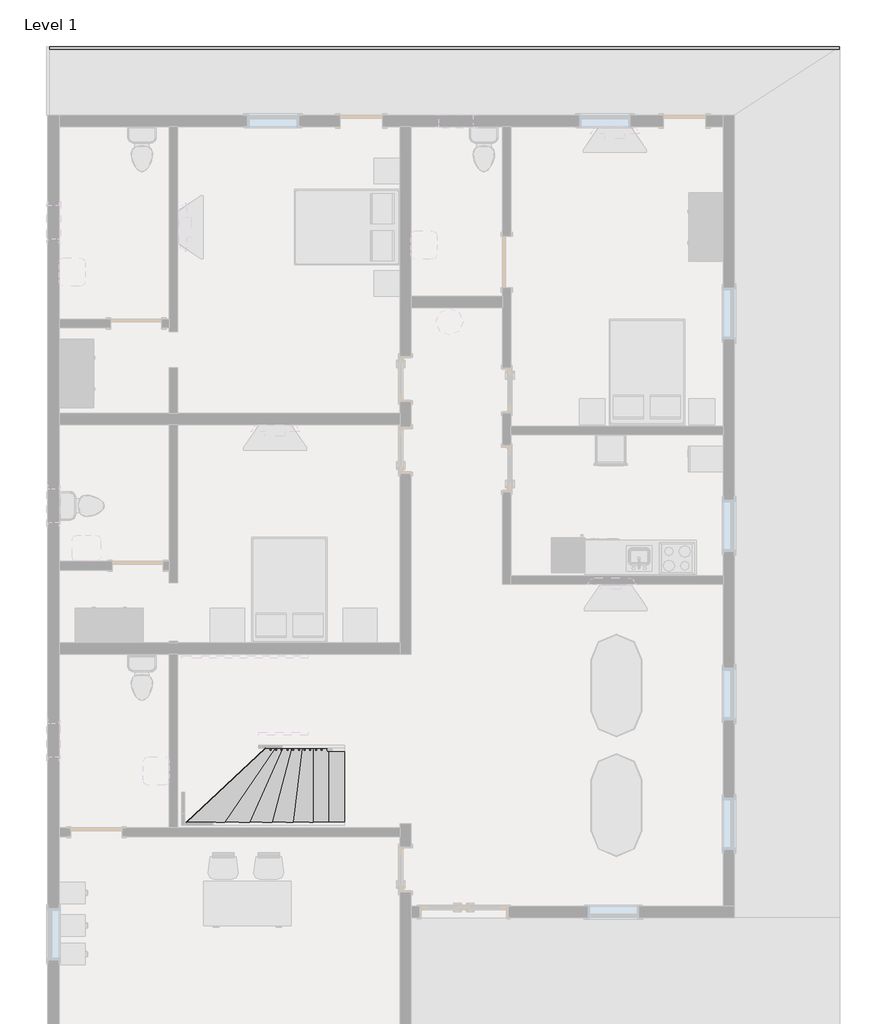
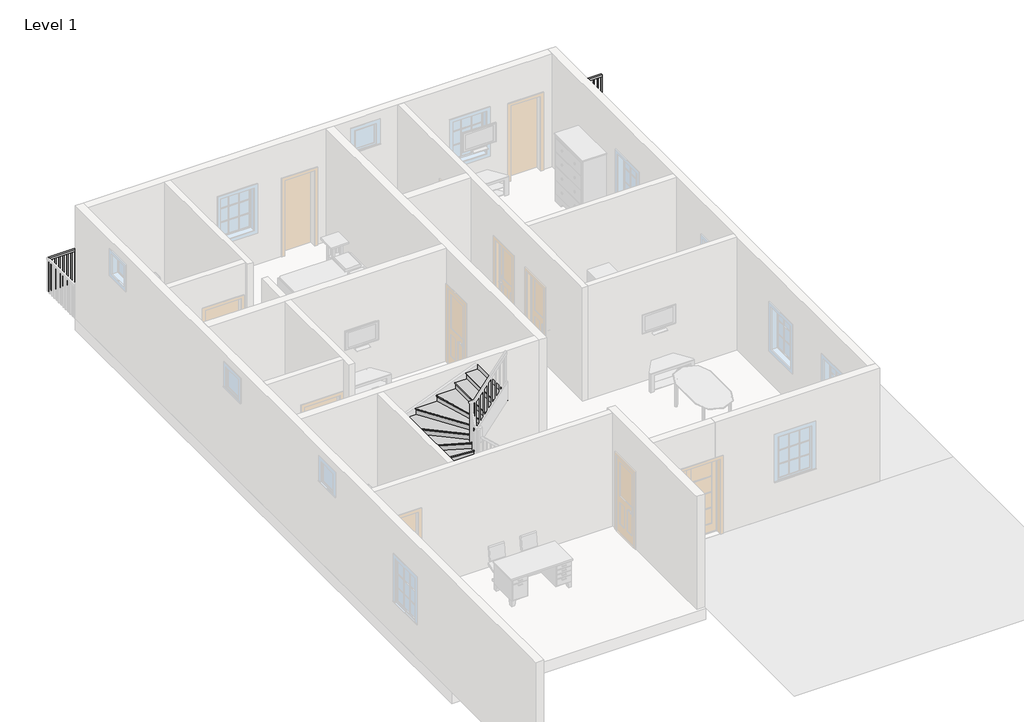
# One storey, part 3 of 4: 1 railing, 1 stair flight.
"""IFC4 building model written with IfcOpenShell, lengths in millimetres."""

from ifc_helpers import new_model, si_unit, frame, origin, origin_with_axes, place, context, project, spatial, polyline, outline, extrude, transform, mapped, element, save
from components import stair_flight_ec2dc638

model = new_model("IFC4")

# Units and contexts
model_context = context("Model", 3, world=origin())
ifc_project = project(units=[si_unit("LENGTHUNIT", "METRE", prefix="MILLI")], contexts=[model_context])

# Site, building, storey
site = spatial("IfcSite", under=ifc_project)
building = spatial("IfcBuilding", under=site)
storey = spatial("IfcBuildingStorey", under=building, Name="Level 1", Elevation=0.0)

# Railing
placement = place(None, origin())
element("IfcRailing", 1, ObjectType="Handrail - Rectangular", at=placement, inside=storey, context=model_context, shape_type="SweptSolid", body=[
    extrude(outline(polyline([(8571.673647, 10436.3488108), (8571.673647, 10385.5488108), (-5525.326353, 10385.5488108), (-5525.326353, 10436.3488108), (8571.673647, 10436.3488108)])), frame((0.0, 0.0, 863.6), z_axis=(0.0, 0.0, 1.0), x_axis=(1.0, 0.0, 0.0)), (0.0, 0.0, 1.0), 50.8),
    extrude(outline(polyline([(-5439.601353, 10420.4738108), (-5439.601353, 10401.4238108), (-5458.651353, 10401.4238108), (-5458.651353, 10420.4738108), (-5439.601353, 10420.4738108)])), origin_with_axes(), (0.0, 0.0, 1.0), 863.6),
    extrude(outline(polyline([(-5338.001353, 10420.4738108), (-5338.001353, 10401.4238108), (-5357.051353, 10401.4238108), (-5357.051353, 10420.4738108), (-5338.001353, 10420.4738108)])), origin_with_axes(), (0.0, 0.0, 1.0), 863.6),
    extrude(outline(polyline([(-5236.401353, 10420.4738108), (-5236.401353, 10401.4238108), (-5255.451353, 10401.4238108), (-5255.451353, 10420.4738108), (-5236.401353, 10420.4738108)])), origin_with_axes(), (0.0, 0.0, 1.0), 863.6),
    extrude(outline(polyline([(-5134.801353, 10420.4738108), (-5134.801353, 10401.4238108), (-5153.851353, 10401.4238108), (-5153.851353, 10420.4738108), (-5134.801353, 10420.4738108)])), origin_with_axes(), (0.0, 0.0, 1.0), 863.6),
    extrude(outline(polyline([(-5033.201353, 10420.4738108), (-5033.201353, 10401.4238108), (-5052.251353, 10401.4238108), (-5052.251353, 10420.4738108), (-5033.201353, 10420.4738108)])), origin_with_axes(), (0.0, 0.0, 1.0), 863.6),
    extrude(outline(polyline([(-4931.601353, 10420.4738108), (-4931.601353, 10401.4238108), (-4950.651353, 10401.4238108), (-4950.651353, 10420.4738108), (-4931.601353, 10420.4738108)])), origin_with_axes(), (0.0, 0.0, 1.0), 863.6),
    extrude(outline(polyline([(-4830.001353, 10420.4738108), (-4830.001353, 10401.4238108), (-4849.051353, 10401.4238108), (-4849.051353, 10420.4738108), (-4830.001353, 10420.4738108)])), origin_with_axes(), (0.0, 0.0, 1.0), 863.6),
    extrude(outline(polyline([(-4728.401353, 10420.4738108), (-4728.401353, 10401.4238108), (-4747.451353, 10401.4238108), (-4747.451353, 10420.4738108), (-4728.401353, 10420.4738108)])), origin_with_axes(), (0.0, 0.0, 1.0), 863.6),
    extrude(outline(polyline([(-4626.801353, 10420.4738108), (-4626.801353, 10401.4238108), (-4645.851353, 10401.4238108), (-4645.851353, 10420.4738108), (-4626.801353, 10420.4738108)])), origin_with_axes(), (0.0, 0.0, 1.0), 863.6),
    extrude(outline(polyline([(-4525.201353, 10420.4738108), (-4525.201353, 10401.4238108), (-4544.251353, 10401.4238108), (-4544.251353, 10420.4738108), (-4525.201353, 10420.4738108)])), origin_with_axes(), (0.0, 0.0, 1.0), 863.6),
    extrude(outline(polyline([(-4423.601353, 10420.4738108), (-4423.601353, 10401.4238108), (-4442.651353, 10401.4238108), (-4442.651353, 10420.4738108), (-4423.601353, 10420.4738108)])), origin_with_axes(), (0.0, 0.0, 1.0), 863.6),
    extrude(outline(polyline([(-4322.001353, 10420.4738108), (-4322.001353, 10401.4238108), (-4341.051353, 10401.4238108), (-4341.051353, 10420.4738108), (-4322.001353, 10420.4738108)])), origin_with_axes(), (0.0, 0.0, 1.0), 863.6),
    extrude(outline(polyline([(-4220.401353, 10420.4738108), (-4220.401353, 10401.4238108), (-4239.451353, 10401.4238108), (-4239.451353, 10420.4738108), (-4220.401353, 10420.4738108)])), origin_with_axes(), (0.0, 0.0, 1.0), 863.6),
    extrude(outline(polyline([(-4118.801353, 10420.4738108), (-4118.801353, 10401.4238108), (-4137.851353, 10401.4238108), (-4137.851353, 10420.4738108), (-4118.801353, 10420.4738108)])), origin_with_axes(), (0.0, 0.0, 1.0), 863.6),
    extrude(outline(polyline([(-4017.201353, 10420.4738108), (-4017.201353, 10401.4238108), (-4036.251353, 10401.4238108), (-4036.251353, 10420.4738108), (-4017.201353, 10420.4738108)])), origin_with_axes(), (0.0, 0.0, 1.0), 863.6),
    extrude(outline(polyline([(-3915.601353, 10420.4738108), (-3915.601353, 10401.4238108), (-3934.651353, 10401.4238108), (-3934.651353, 10420.4738108), (-3915.601353, 10420.4738108)])), origin_with_axes(), (0.0, 0.0, 1.0), 863.6),
    extrude(outline(polyline([(-3814.001353, 10420.4738108), (-3814.001353, 10401.4238108), (-3833.051353, 10401.4238108), (-3833.051353, 10420.4738108), (-3814.001353, 10420.4738108)])), origin_with_axes(), (0.0, 0.0, 1.0), 863.6),
    extrude(outline(polyline([(-3712.401353, 10420.4738108), (-3712.401353, 10401.4238108), (-3731.451353, 10401.4238108), (-3731.451353, 10420.4738108), (-3712.401353, 10420.4738108)])), origin_with_axes(), (0.0, 0.0, 1.0), 863.6),
    extrude(outline(polyline([(-3610.801353, 10420.4738108), (-3610.801353, 10401.4238108), (-3629.851353, 10401.4238108), (-3629.851353, 10420.4738108), (-3610.801353, 10420.4738108)])), origin_with_axes(), (0.0, 0.0, 1.0), 863.6),
    extrude(outline(polyline([(-3509.201353, 10420.4738108), (-3509.201353, 10401.4238108), (-3528.251353, 10401.4238108), (-3528.251353, 10420.4738108), (-3509.201353, 10420.4738108)])), origin_with_axes(), (0.0, 0.0, 1.0), 863.6),
    extrude(outline(polyline([(-3407.601353, 10420.4738108), (-3407.601353, 10401.4238108), (-3426.651353, 10401.4238108), (-3426.651353, 10420.4738108), (-3407.601353, 10420.4738108)])), origin_with_axes(), (0.0, 0.0, 1.0), 863.6),
    extrude(outline(polyline([(-3306.001353, 10420.4738108), (-3306.001353, 10401.4238108), (-3325.051353, 10401.4238108), (-3325.051353, 10420.4738108), (-3306.001353, 10420.4738108)])), origin_with_axes(), (0.0, 0.0, 1.0), 863.6),
    extrude(outline(polyline([(-3204.401353, 10420.4738108), (-3204.401353, 10401.4238108), (-3223.451353, 10401.4238108), (-3223.451353, 10420.4738108), (-3204.401353, 10420.4738108)])), origin_with_axes(), (0.0, 0.0, 1.0), 863.6),
    extrude(outline(polyline([(-3102.801353, 10420.4738108), (-3102.801353, 10401.4238108), (-3121.851353, 10401.4238108), (-3121.851353, 10420.4738108), (-3102.801353, 10420.4738108)])), origin_with_axes(), (0.0, 0.0, 1.0), 863.6),
    extrude(outline(polyline([(-3001.201353, 10420.4738108), (-3001.201353, 10401.4238108), (-3020.251353, 10401.4238108), (-3020.251353, 10420.4738108), (-3001.201353, 10420.4738108)])), origin_with_axes(), (0.0, 0.0, 1.0), 863.6),
    extrude(outline(polyline([(-2899.601353, 10420.4738108), (-2899.601353, 10401.4238108), (-2918.651353, 10401.4238108), (-2918.651353, 10420.4738108), (-2899.601353, 10420.4738108)])), origin_with_axes(), (0.0, 0.0, 1.0), 863.6),
    extrude(outline(polyline([(-2798.001353, 10420.4738108), (-2798.001353, 10401.4238108), (-2817.051353, 10401.4238108), (-2817.051353, 10420.4738108), (-2798.001353, 10420.4738108)])), origin_with_axes(), (0.0, 0.0, 1.0), 863.6),
    extrude(outline(polyline([(-2696.401353, 10420.4738108), (-2696.401353, 10401.4238108), (-2715.451353, 10401.4238108), (-2715.451353, 10420.4738108), (-2696.401353, 10420.4738108)])), origin_with_axes(), (0.0, 0.0, 1.0), 863.6),
    extrude(outline(polyline([(-2594.801353, 10420.4738108), (-2594.801353, 10401.4238108), (-2613.851353, 10401.4238108), (-2613.851353, 10420.4738108), (-2594.801353, 10420.4738108)])), origin_with_axes(), (0.0, 0.0, 1.0), 863.6),
    extrude(outline(polyline([(-2493.201353, 10420.4738108), (-2493.201353, 10401.4238108), (-2512.251353, 10401.4238108), (-2512.251353, 10420.4738108), (-2493.201353, 10420.4738108)])), origin_with_axes(), (0.0, 0.0, 1.0), 863.6),
    extrude(outline(polyline([(-2391.601353, 10420.4738108), (-2391.601353, 10401.4238108), (-2410.651353, 10401.4238108), (-2410.651353, 10420.4738108), (-2391.601353, 10420.4738108)])), origin_with_axes(), (0.0, 0.0, 1.0), 863.6),
    extrude(outline(polyline([(-2290.001353, 10420.4738108), (-2290.001353, 10401.4238108), (-2309.051353, 10401.4238108), (-2309.051353, 10420.4738108), (-2290.001353, 10420.4738108)])), origin_with_axes(), (0.0, 0.0, 1.0), 863.6),
    extrude(outline(polyline([(-2188.401353, 10420.4738108), (-2188.401353, 10401.4238108), (-2207.451353, 10401.4238108), (-2207.451353, 10420.4738108), (-2188.401353, 10420.4738108)])), origin_with_axes(), (0.0, 0.0, 1.0), 863.6),
    extrude(outline(polyline([(-2086.801353, 10420.4738108), (-2086.801353, 10401.4238108), (-2105.851353, 10401.4238108), (-2105.851353, 10420.4738108), (-2086.801353, 10420.4738108)])), origin_with_axes(), (0.0, 0.0, 1.0), 863.6),
    extrude(outline(polyline([(-1985.201353, 10420.4738108), (-1985.201353, 10401.4238108), (-2004.251353, 10401.4238108), (-2004.251353, 10420.4738108), (-1985.201353, 10420.4738108)])), origin_with_axes(), (0.0, 0.0, 1.0), 863.6),
    extrude(outline(polyline([(-1883.601353, 10420.4738108), (-1883.601353, 10401.4238108), (-1902.651353, 10401.4238108), (-1902.651353, 10420.4738108), (-1883.601353, 10420.4738108)])), origin_with_axes(), (0.0, 0.0, 1.0), 863.6),
    extrude(outline(polyline([(-1782.001353, 10420.4738108), (-1782.001353, 10401.4238108), (-1801.051353, 10401.4238108), (-1801.051353, 10420.4738108), (-1782.001353, 10420.4738108)])), origin_with_axes(), (0.0, 0.0, 1.0), 863.6),
    extrude(outline(polyline([(-1680.401353, 10420.4738108), (-1680.401353, 10401.4238108), (-1699.451353, 10401.4238108), (-1699.451353, 10420.4738108), (-1680.401353, 10420.4738108)])), origin_with_axes(), (0.0, 0.0, 1.0), 863.6),
    extrude(outline(polyline([(-1578.801353, 10420.4738108), (-1578.801353, 10401.4238108), (-1597.851353, 10401.4238108), (-1597.851353, 10420.4738108), (-1578.801353, 10420.4738108)])), origin_with_axes(), (0.0, 0.0, 1.0), 863.6),
    extrude(outline(polyline([(-1477.201353, 10420.4738108), (-1477.201353, 10401.4238108), (-1496.251353, 10401.4238108), (-1496.251353, 10420.4738108), (-1477.201353, 10420.4738108)])), origin_with_axes(), (0.0, 0.0, 1.0), 863.6),
    extrude(outline(polyline([(-1375.601353, 10420.4738108), (-1375.601353, 10401.4238108), (-1394.651353, 10401.4238108), (-1394.651353, 10420.4738108), (-1375.601353, 10420.4738108)])), origin_with_axes(), (0.0, 0.0, 1.0), 863.6),
    extrude(outline(polyline([(-1274.001353, 10420.4738108), (-1274.001353, 10401.4238108), (-1293.051353, 10401.4238108), (-1293.051353, 10420.4738108), (-1274.001353, 10420.4738108)])), origin_with_axes(), (0.0, 0.0, 1.0), 863.6),
    extrude(outline(polyline([(-1172.401353, 10420.4738108), (-1172.401353, 10401.4238108), (-1191.451353, 10401.4238108), (-1191.451353, 10420.4738108), (-1172.401353, 10420.4738108)])), origin_with_axes(), (0.0, 0.0, 1.0), 863.6),
    extrude(outline(polyline([(-1070.801353, 10420.4738108), (-1070.801353, 10401.4238108), (-1089.851353, 10401.4238108), (-1089.851353, 10420.4738108), (-1070.801353, 10420.4738108)])), origin_with_axes(), (0.0, 0.0, 1.0), 863.6),
    extrude(outline(polyline([(-969.201353, 10420.4738108), (-969.201353, 10401.4238108), (-988.251353, 10401.4238108), (-988.251353, 10420.4738108), (-969.201353, 10420.4738108)])), origin_with_axes(), (0.0, 0.0, 1.0), 863.6),
    extrude(outline(polyline([(-867.601353, 10420.4738108), (-867.601353, 10401.4238108), (-886.651353, 10401.4238108), (-886.651353, 10420.4738108), (-867.601353, 10420.4738108)])), origin_with_axes(), (0.0, 0.0, 1.0), 863.6),
    extrude(outline(polyline([(-766.001353, 10420.4738108), (-766.001353, 10401.4238108), (-785.051353, 10401.4238108), (-785.051353, 10420.4738108), (-766.001353, 10420.4738108)])), origin_with_axes(), (0.0, 0.0, 1.0), 863.6),
    extrude(outline(polyline([(-664.401353, 10420.4738108), (-664.401353, 10401.4238108), (-683.451353, 10401.4238108), (-683.451353, 10420.4738108), (-664.401353, 10420.4738108)])), origin_with_axes(), (0.0, 0.0, 1.0), 863.6),
    extrude(outline(polyline([(-562.801353, 10420.4738108), (-562.801353, 10401.4238108), (-581.851353, 10401.4238108), (-581.851353, 10420.4738108), (-562.801353, 10420.4738108)])), origin_with_axes(), (0.0, 0.0, 1.0), 863.6),
    extrude(outline(polyline([(-461.201353, 10420.4738108), (-461.201353, 10401.4238108), (-480.251353, 10401.4238108), (-480.251353, 10420.4738108), (-461.201353, 10420.4738108)])), origin_with_axes(), (0.0, 0.0, 1.0), 863.6),
    extrude(outline(polyline([(-359.601353, 10420.4738108), (-359.601353, 10401.4238108), (-378.651353, 10401.4238108), (-378.651353, 10420.4738108), (-359.601353, 10420.4738108)])), origin_with_axes(), (0.0, 0.0, 1.0), 863.6),
    extrude(outline(polyline([(-258.001353, 10420.4738108), (-258.001353, 10401.4238108), (-277.051353, 10401.4238108), (-277.051353, 10420.4738108), (-258.001353, 10420.4738108)])), origin_with_axes(), (0.0, 0.0, 1.0), 863.6),
    extrude(outline(polyline([(-156.401353, 10420.4738108), (-156.401353, 10401.4238108), (-175.451353, 10401.4238108), (-175.451353, 10420.4738108), (-156.401353, 10420.4738108)])), origin_with_axes(), (0.0, 0.0, 1.0), 863.6),
    extrude(outline(polyline([(-54.801353, 10420.4738108), (-54.801353, 10401.4238108), (-73.851353, 10401.4238108), (-73.851353, 10420.4738108), (-54.801353, 10420.4738108)])), origin_with_axes(), (0.0, 0.0, 1.0), 863.6),
    extrude(outline(polyline([(46.798647, 10420.4738108), (46.798647, 10401.4238108), (27.748647, 10401.4238108), (27.748647, 10420.4738108), (46.798647, 10420.4738108)])), origin_with_axes(), (0.0, 0.0, 1.0), 863.6),
    extrude(outline(polyline([(148.398647, 10420.4738108), (148.398647, 10401.4238108), (129.348647, 10401.4238108), (129.348647, 10420.4738108), (148.398647, 10420.4738108)])), origin_with_axes(), (0.0, 0.0, 1.0), 863.6),
    extrude(outline(polyline([(249.998647, 10420.4738108), (249.998647, 10401.4238108), (230.948647, 10401.4238108), (230.948647, 10420.4738108), (249.998647, 10420.4738108)])), origin_with_axes(), (0.0, 0.0, 1.0), 863.6),
    extrude(outline(polyline([(351.598647, 10420.4738108), (351.598647, 10401.4238108), (332.548647, 10401.4238108), (332.548647, 10420.4738108), (351.598647, 10420.4738108)])), origin_with_axes(), (0.0, 0.0, 1.0), 863.6),
    extrude(outline(polyline([(453.198647, 10420.4738108), (453.198647, 10401.4238108), (434.148647, 10401.4238108), (434.148647, 10420.4738108), (453.198647, 10420.4738108)])), origin_with_axes(), (0.0, 0.0, 1.0), 863.6),
    extrude(outline(polyline([(554.798647, 10420.4738108), (554.798647, 10401.4238108), (535.748647, 10401.4238108), (535.748647, 10420.4738108), (554.798647, 10420.4738108)])), origin_with_axes(), (0.0, 0.0, 1.0), 863.6),
    extrude(outline(polyline([(656.398647, 10420.4738108), (656.398647, 10401.4238108), (637.348647, 10401.4238108), (637.348647, 10420.4738108), (656.398647, 10420.4738108)])), origin_with_axes(), (0.0, 0.0, 1.0), 863.6),
    extrude(outline(polyline([(757.998647, 10420.4738108), (757.998647, 10401.4238108), (738.948647, 10401.4238108), (738.948647, 10420.4738108), (757.998647, 10420.4738108)])), origin_with_axes(), (0.0, 0.0, 1.0), 863.6),
    extrude(outline(polyline([(859.598647, 10420.4738108), (859.598647, 10401.4238108), (840.548647, 10401.4238108), (840.548647, 10420.4738108), (859.598647, 10420.4738108)])), origin_with_axes(), (0.0, 0.0, 1.0), 863.6),
    extrude(outline(polyline([(961.198647, 10420.4738108), (961.198647, 10401.4238108), (942.148647, 10401.4238108), (942.148647, 10420.4738108), (961.198647, 10420.4738108)])), origin_with_axes(), (0.0, 0.0, 1.0), 863.6),
    extrude(outline(polyline([(1062.798647, 10420.4738108), (1062.798647, 10401.4238108), (1043.748647, 10401.4238108), (1043.748647, 10420.4738108), (1062.798647, 10420.4738108)])), origin_with_axes(), (0.0, 0.0, 1.0), 863.6),
    extrude(outline(polyline([(1164.398647, 10420.4738108), (1164.398647, 10401.4238108), (1145.348647, 10401.4238108), (1145.348647, 10420.4738108), (1164.398647, 10420.4738108)])), origin_with_axes(), (0.0, 0.0, 1.0), 863.6),
    extrude(outline(polyline([(1265.998647, 10420.4738108), (1265.998647, 10401.4238108), (1246.948647, 10401.4238108), (1246.948647, 10420.4738108), (1265.998647, 10420.4738108)])), origin_with_axes(), (0.0, 0.0, 1.0), 863.6),
    extrude(outline(polyline([(1367.598647, 10420.4738108), (1367.598647, 10401.4238108), (1348.548647, 10401.4238108), (1348.548647, 10420.4738108), (1367.598647, 10420.4738108)])), origin_with_axes(), (0.0, 0.0, 1.0), 863.6),
    extrude(outline(polyline([(1469.198647, 10420.4738108), (1469.198647, 10401.4238108), (1450.148647, 10401.4238108), (1450.148647, 10420.4738108), (1469.198647, 10420.4738108)])), origin_with_axes(), (0.0, 0.0, 1.0), 863.6),
    extrude(outline(polyline([(1570.798647, 10420.4738108), (1570.798647, 10401.4238108), (1551.748647, 10401.4238108), (1551.748647, 10420.4738108), (1570.798647, 10420.4738108)])), origin_with_axes(), (0.0, 0.0, 1.0), 863.6),
    extrude(outline(polyline([(1672.398647, 10420.4738108), (1672.398647, 10401.4238108), (1653.348647, 10401.4238108), (1653.348647, 10420.4738108), (1672.398647, 10420.4738108)])), origin_with_axes(), (0.0, 0.0, 1.0), 863.6),
    extrude(outline(polyline([(1773.998647, 10420.4738108), (1773.998647, 10401.4238108), (1754.948647, 10401.4238108), (1754.948647, 10420.4738108), (1773.998647, 10420.4738108)])), origin_with_axes(), (0.0, 0.0, 1.0), 863.6),
    extrude(outline(polyline([(1875.598647, 10420.4738108), (1875.598647, 10401.4238108), (1856.548647, 10401.4238108), (1856.548647, 10420.4738108), (1875.598647, 10420.4738108)])), origin_with_axes(), (0.0, 0.0, 1.0), 863.6),
    extrude(outline(polyline([(1977.198647, 10420.4738108), (1977.198647, 10401.4238108), (1958.148647, 10401.4238108), (1958.148647, 10420.4738108), (1977.198647, 10420.4738108)])), origin_with_axes(), (0.0, 0.0, 1.0), 863.6),
    extrude(outline(polyline([(2078.798647, 10420.4738108), (2078.798647, 10401.4238108), (2059.748647, 10401.4238108), (2059.748647, 10420.4738108), (2078.798647, 10420.4738108)])), origin_with_axes(), (0.0, 0.0, 1.0), 863.6),
    extrude(outline(polyline([(2180.398647, 10420.4738108), (2180.398647, 10401.4238108), (2161.348647, 10401.4238108), (2161.348647, 10420.4738108), (2180.398647, 10420.4738108)])), origin_with_axes(), (0.0, 0.0, 1.0), 863.6),
    extrude(outline(polyline([(2281.998647, 10420.4738108), (2281.998647, 10401.4238108), (2262.948647, 10401.4238108), (2262.948647, 10420.4738108), (2281.998647, 10420.4738108)])), origin_with_axes(), (0.0, 0.0, 1.0), 863.6),
    extrude(outline(polyline([(2383.598647, 10420.4738108), (2383.598647, 10401.4238108), (2364.548647, 10401.4238108), (2364.548647, 10420.4738108), (2383.598647, 10420.4738108)])), origin_with_axes(), (0.0, 0.0, 1.0), 863.6),
    extrude(outline(polyline([(2485.198647, 10420.4738108), (2485.198647, 10401.4238108), (2466.148647, 10401.4238108), (2466.148647, 10420.4738108), (2485.198647, 10420.4738108)])), origin_with_axes(), (0.0, 0.0, 1.0), 863.6),
    extrude(outline(polyline([(2586.798647, 10420.4738108), (2586.798647, 10401.4238108), (2567.748647, 10401.4238108), (2567.748647, 10420.4738108), (2586.798647, 10420.4738108)])), origin_with_axes(), (0.0, 0.0, 1.0), 863.6),
    extrude(outline(polyline([(2688.398647, 10420.4738108), (2688.398647, 10401.4238108), (2669.348647, 10401.4238108), (2669.348647, 10420.4738108), (2688.398647, 10420.4738108)])), origin_with_axes(), (0.0, 0.0, 1.0), 863.6),
    extrude(outline(polyline([(2789.998647, 10420.4738108), (2789.998647, 10401.4238108), (2770.948647, 10401.4238108), (2770.948647, 10420.4738108), (2789.998647, 10420.4738108)])), origin_with_axes(), (0.0, 0.0, 1.0), 863.6),
    extrude(outline(polyline([(2891.598647, 10420.4738108), (2891.598647, 10401.4238108), (2872.548647, 10401.4238108), (2872.548647, 10420.4738108), (2891.598647, 10420.4738108)])), origin_with_axes(), (0.0, 0.0, 1.0), 863.6),
    extrude(outline(polyline([(2993.198647, 10420.4738108), (2993.198647, 10401.4238108), (2974.148647, 10401.4238108), (2974.148647, 10420.4738108), (2993.198647, 10420.4738108)])), origin_with_axes(), (0.0, 0.0, 1.0), 863.6),
    extrude(outline(polyline([(3094.798647, 10420.4738108), (3094.798647, 10401.4238108), (3075.748647, 10401.4238108), (3075.748647, 10420.4738108), (3094.798647, 10420.4738108)])), origin_with_axes(), (0.0, 0.0, 1.0), 863.6),
    extrude(outline(polyline([(3196.398647, 10420.4738108), (3196.398647, 10401.4238108), (3177.348647, 10401.4238108), (3177.348647, 10420.4738108), (3196.398647, 10420.4738108)])), origin_with_axes(), (0.0, 0.0, 1.0), 863.6),
    extrude(outline(polyline([(3297.998647, 10420.4738108), (3297.998647, 10401.4238108), (3278.948647, 10401.4238108), (3278.948647, 10420.4738108), (3297.998647, 10420.4738108)])), origin_with_axes(), (0.0, 0.0, 1.0), 863.6),
    extrude(outline(polyline([(3399.598647, 10420.4738108), (3399.598647, 10401.4238108), (3380.548647, 10401.4238108), (3380.548647, 10420.4738108), (3399.598647, 10420.4738108)])), origin_with_axes(), (0.0, 0.0, 1.0), 863.6),
    extrude(outline(polyline([(3501.198647, 10420.4738108), (3501.198647, 10401.4238108), (3482.148647, 10401.4238108), (3482.148647, 10420.4738108), (3501.198647, 10420.4738108)])), origin_with_axes(), (0.0, 0.0, 1.0), 863.6),
    extrude(outline(polyline([(3602.798647, 10420.4738108), (3602.798647, 10401.4238108), (3583.748647, 10401.4238108), (3583.748647, 10420.4738108), (3602.798647, 10420.4738108)])), origin_with_axes(), (0.0, 0.0, 1.0), 863.6),
    extrude(outline(polyline([(3704.398647, 10420.4738108), (3704.398647, 10401.4238108), (3685.348647, 10401.4238108), (3685.348647, 10420.4738108), (3704.398647, 10420.4738108)])), origin_with_axes(), (0.0, 0.0, 1.0), 863.6),
    extrude(outline(polyline([(3805.998647, 10420.4738108), (3805.998647, 10401.4238108), (3786.948647, 10401.4238108), (3786.948647, 10420.4738108), (3805.998647, 10420.4738108)])), origin_with_axes(), (0.0, 0.0, 1.0), 863.6),
    extrude(outline(polyline([(3907.598647, 10420.4738108), (3907.598647, 10401.4238108), (3888.548647, 10401.4238108), (3888.548647, 10420.4738108), (3907.598647, 10420.4738108)])), origin_with_axes(), (0.0, 0.0, 1.0), 863.6),
    extrude(outline(polyline([(4009.198647, 10420.4738108), (4009.198647, 10401.4238108), (3990.148647, 10401.4238108), (3990.148647, 10420.4738108), (4009.198647, 10420.4738108)])), origin_with_axes(), (0.0, 0.0, 1.0), 863.6),
    extrude(outline(polyline([(4110.798647, 10420.4738108), (4110.798647, 10401.4238108), (4091.748647, 10401.4238108), (4091.748647, 10420.4738108), (4110.798647, 10420.4738108)])), origin_with_axes(), (0.0, 0.0, 1.0), 863.6),
    extrude(outline(polyline([(4212.398647, 10420.4738108), (4212.398647, 10401.4238108), (4193.348647, 10401.4238108), (4193.348647, 10420.4738108), (4212.398647, 10420.4738108)])), origin_with_axes(), (0.0, 0.0, 1.0), 863.6),
    extrude(outline(polyline([(4313.998647, 10420.4738108), (4313.998647, 10401.4238108), (4294.948647, 10401.4238108), (4294.948647, 10420.4738108), (4313.998647, 10420.4738108)])), origin_with_axes(), (0.0, 0.0, 1.0), 863.6),
    extrude(outline(polyline([(4415.598647, 10420.4738108), (4415.598647, 10401.4238108), (4396.548647, 10401.4238108), (4396.548647, 10420.4738108), (4415.598647, 10420.4738108)])), origin_with_axes(), (0.0, 0.0, 1.0), 863.6),
    extrude(outline(polyline([(4517.198647, 10420.4738108), (4517.198647, 10401.4238108), (4498.148647, 10401.4238108), (4498.148647, 10420.4738108), (4517.198647, 10420.4738108)])), origin_with_axes(), (0.0, 0.0, 1.0), 863.6),
    extrude(outline(polyline([(4618.798647, 10420.4738108), (4618.798647, 10401.4238108), (4599.748647, 10401.4238108), (4599.748647, 10420.4738108), (4618.798647, 10420.4738108)])), origin_with_axes(), (0.0, 0.0, 1.0), 863.6),
    extrude(outline(polyline([(4720.398647, 10420.4738108), (4720.398647, 10401.4238108), (4701.348647, 10401.4238108), (4701.348647, 10420.4738108), (4720.398647, 10420.4738108)])), origin_with_axes(), (0.0, 0.0, 1.0), 863.6),
    extrude(outline(polyline([(4821.998647, 10420.4738108), (4821.998647, 10401.4238108), (4802.948647, 10401.4238108), (4802.948647, 10420.4738108), (4821.998647, 10420.4738108)])), origin_with_axes(), (0.0, 0.0, 1.0), 863.6),
    extrude(outline(polyline([(4923.598647, 10420.4738108), (4923.598647, 10401.4238108), (4904.548647, 10401.4238108), (4904.548647, 10420.4738108), (4923.598647, 10420.4738108)])), origin_with_axes(), (0.0, 0.0, 1.0), 863.6),
    extrude(outline(polyline([(5025.198647, 10420.4738108), (5025.198647, 10401.4238108), (5006.148647, 10401.4238108), (5006.148647, 10420.4738108), (5025.198647, 10420.4738108)])), origin_with_axes(), (0.0, 0.0, 1.0), 863.6),
    extrude(outline(polyline([(5126.798647, 10420.4738108), (5126.798647, 10401.4238108), (5107.748647, 10401.4238108), (5107.748647, 10420.4738108), (5126.798647, 10420.4738108)])), origin_with_axes(), (0.0, 0.0, 1.0), 863.6),
    extrude(outline(polyline([(5228.398647, 10420.4738108), (5228.398647, 10401.4238108), (5209.348647, 10401.4238108), (5209.348647, 10420.4738108), (5228.398647, 10420.4738108)])), origin_with_axes(), (0.0, 0.0, 1.0), 863.6),
    extrude(outline(polyline([(5329.998647, 10420.4738108), (5329.998647, 10401.4238108), (5310.948647, 10401.4238108), (5310.948647, 10420.4738108), (5329.998647, 10420.4738108)])), origin_with_axes(), (0.0, 0.0, 1.0), 863.6),
    extrude(outline(polyline([(5431.598647, 10420.4738108), (5431.598647, 10401.4238108), (5412.548647, 10401.4238108), (5412.548647, 10420.4738108), (5431.598647, 10420.4738108)])), origin_with_axes(), (0.0, 0.0, 1.0), 863.6),
    extrude(outline(polyline([(5533.198647, 10420.4738108), (5533.198647, 10401.4238108), (5514.148647, 10401.4238108), (5514.148647, 10420.4738108), (5533.198647, 10420.4738108)])), origin_with_axes(), (0.0, 0.0, 1.0), 863.6),
    extrude(outline(polyline([(5634.798647, 10420.4738108), (5634.798647, 10401.4238108), (5615.748647, 10401.4238108), (5615.748647, 10420.4738108), (5634.798647, 10420.4738108)])), origin_with_axes(), (0.0, 0.0, 1.0), 863.6),
    extrude(outline(polyline([(5736.398647, 10420.4738108), (5736.398647, 10401.4238108), (5717.348647, 10401.4238108), (5717.348647, 10420.4738108), (5736.398647, 10420.4738108)])), origin_with_axes(), (0.0, 0.0, 1.0), 863.6),
    extrude(outline(polyline([(5837.998647, 10420.4738108), (5837.998647, 10401.4238108), (5818.948647, 10401.4238108), (5818.948647, 10420.4738108), (5837.998647, 10420.4738108)])), origin_with_axes(), (0.0, 0.0, 1.0), 863.6),
    extrude(outline(polyline([(5939.598647, 10420.4738108), (5939.598647, 10401.4238108), (5920.548647, 10401.4238108), (5920.548647, 10420.4738108), (5939.598647, 10420.4738108)])), origin_with_axes(), (0.0, 0.0, 1.0), 863.6),
    extrude(outline(polyline([(6041.198647, 10420.4738108), (6041.198647, 10401.4238108), (6022.148647, 10401.4238108), (6022.148647, 10420.4738108), (6041.198647, 10420.4738108)])), origin_with_axes(), (0.0, 0.0, 1.0), 863.6),
    extrude(outline(polyline([(6142.798647, 10420.4738108), (6142.798647, 10401.4238108), (6123.748647, 10401.4238108), (6123.748647, 10420.4738108), (6142.798647, 10420.4738108)])), origin_with_axes(), (0.0, 0.0, 1.0), 863.6),
    extrude(outline(polyline([(6244.398647, 10420.4738108), (6244.398647, 10401.4238108), (6225.348647, 10401.4238108), (6225.348647, 10420.4738108), (6244.398647, 10420.4738108)])), origin_with_axes(), (0.0, 0.0, 1.0), 863.6),
    extrude(outline(polyline([(6345.998647, 10420.4738108), (6345.998647, 10401.4238108), (6326.948647, 10401.4238108), (6326.948647, 10420.4738108), (6345.998647, 10420.4738108)])), origin_with_axes(), (0.0, 0.0, 1.0), 863.6),
    extrude(outline(polyline([(6447.598647, 10420.4738108), (6447.598647, 10401.4238108), (6428.548647, 10401.4238108), (6428.548647, 10420.4738108), (6447.598647, 10420.4738108)])), origin_with_axes(), (0.0, 0.0, 1.0), 863.6),
    extrude(outline(polyline([(6549.198647, 10420.4738108), (6549.198647, 10401.4238108), (6530.148647, 10401.4238108), (6530.148647, 10420.4738108), (6549.198647, 10420.4738108)])), origin_with_axes(), (0.0, 0.0, 1.0), 863.6),
    extrude(outline(polyline([(6650.798647, 10420.4738108), (6650.798647, 10401.4238108), (6631.748647, 10401.4238108), (6631.748647, 10420.4738108), (6650.798647, 10420.4738108)])), origin_with_axes(), (0.0, 0.0, 1.0), 863.6),
    extrude(outline(polyline([(6752.398647, 10420.4738108), (6752.398647, 10401.4238108), (6733.348647, 10401.4238108), (6733.348647, 10420.4738108), (6752.398647, 10420.4738108)])), origin_with_axes(), (0.0, 0.0, 1.0), 863.6),
    extrude(outline(polyline([(6853.998647, 10420.4738108), (6853.998647, 10401.4238108), (6834.948647, 10401.4238108), (6834.948647, 10420.4738108), (6853.998647, 10420.4738108)])), origin_with_axes(), (0.0, 0.0, 1.0), 863.6),
    extrude(outline(polyline([(6955.598647, 10420.4738108), (6955.598647, 10401.4238108), (6936.548647, 10401.4238108), (6936.548647, 10420.4738108), (6955.598647, 10420.4738108)])), origin_with_axes(), (0.0, 0.0, 1.0), 863.6),
    extrude(outline(polyline([(7057.198647, 10420.4738108), (7057.198647, 10401.4238108), (7038.148647, 10401.4238108), (7038.148647, 10420.4738108), (7057.198647, 10420.4738108)])), origin_with_axes(), (0.0, 0.0, 1.0), 863.6),
    extrude(outline(polyline([(7158.798647, 10420.4738108), (7158.798647, 10401.4238108), (7139.748647, 10401.4238108), (7139.748647, 10420.4738108), (7158.798647, 10420.4738108)])), origin_with_axes(), (0.0, 0.0, 1.0), 863.6),
    extrude(outline(polyline([(7260.398647, 10420.4738108), (7260.398647, 10401.4238108), (7241.348647, 10401.4238108), (7241.348647, 10420.4738108), (7260.398647, 10420.4738108)])), origin_with_axes(), (0.0, 0.0, 1.0), 863.6),
    extrude(outline(polyline([(7361.998647, 10420.4738108), (7361.998647, 10401.4238108), (7342.948647, 10401.4238108), (7342.948647, 10420.4738108), (7361.998647, 10420.4738108)])), origin_with_axes(), (0.0, 0.0, 1.0), 863.6),
    extrude(outline(polyline([(7463.598647, 10420.4738108), (7463.598647, 10401.4238108), (7444.548647, 10401.4238108), (7444.548647, 10420.4738108), (7463.598647, 10420.4738108)])), origin_with_axes(), (0.0, 0.0, 1.0), 863.6),
    extrude(outline(polyline([(7565.198647, 10420.4738108), (7565.198647, 10401.4238108), (7546.148647, 10401.4238108), (7546.148647, 10420.4738108), (7565.198647, 10420.4738108)])), origin_with_axes(), (0.0, 0.0, 1.0), 863.6),
    extrude(outline(polyline([(7666.798647, 10420.4738108), (7666.798647, 10401.4238108), (7647.748647, 10401.4238108), (7647.748647, 10420.4738108), (7666.798647, 10420.4738108)])), origin_with_axes(), (0.0, 0.0, 1.0), 863.6),
    extrude(outline(polyline([(7768.398647, 10420.4738108), (7768.398647, 10401.4238108), (7749.348647, 10401.4238108), (7749.348647, 10420.4738108), (7768.398647, 10420.4738108)])), origin_with_axes(), (0.0, 0.0, 1.0), 863.6),
    extrude(outline(polyline([(7869.998647, 10420.4738108), (7869.998647, 10401.4238108), (7850.948647, 10401.4238108), (7850.948647, 10420.4738108), (7869.998647, 10420.4738108)])), origin_with_axes(), (0.0, 0.0, 1.0), 863.6),
    extrude(outline(polyline([(7971.598647, 10420.4738108), (7971.598647, 10401.4238108), (7952.548647, 10401.4238108), (7952.548647, 10420.4738108), (7971.598647, 10420.4738108)])), origin_with_axes(), (0.0, 0.0, 1.0), 863.6),
    extrude(outline(polyline([(8073.198647, 10420.4738108), (8073.198647, 10401.4238108), (8054.148647, 10401.4238108), (8054.148647, 10420.4738108), (8073.198647, 10420.4738108)])), origin_with_axes(), (0.0, 0.0, 1.0), 863.6),
    extrude(outline(polyline([(8174.798647, 10420.4738108), (8174.798647, 10401.4238108), (8155.748647, 10401.4238108), (8155.748647, 10420.4738108), (8174.798647, 10420.4738108)])), origin_with_axes(), (0.0, 0.0, 1.0), 863.6),
    extrude(outline(polyline([(8276.398647, 10420.4738108), (8276.398647, 10401.4238108), (8257.348647, 10401.4238108), (8257.348647, 10420.4738108), (8276.398647, 10420.4738108)])), origin_with_axes(), (0.0, 0.0, 1.0), 863.6),
    extrude(outline(polyline([(8377.998647, 10420.4738108), (8377.998647, 10401.4238108), (8358.948647, 10401.4238108), (8358.948647, 10420.4738108), (8377.998647, 10420.4738108)])), origin_with_axes(), (0.0, 0.0, 1.0), 863.6),
    extrude(outline(polyline([(8479.598647, 10420.4738108), (8479.598647, 10401.4238108), (8460.548647, 10401.4238108), (8460.548647, 10420.4738108), (8479.598647, 10420.4738108)])), origin_with_axes(), (0.0, 0.0, 1.0), 863.6),
    extrude(outline(polyline([(-5506.276353, 10420.4738108), (-5506.276353, 10401.4238108), (-5525.326353, 10401.4238108), (-5525.326353, 10420.4738108), (-5506.276353, 10420.4738108)])), origin_with_axes(), (0.0, 0.0, 1.0), 863.6),
    extrude(outline(polyline([(8571.673647, 10420.4738108), (8571.673647, 10401.4238108), (8552.623647, 10401.4238108), (8552.623647, 10420.4738108), (8571.673647, 10420.4738108)])), origin_with_axes(), (0.0, 0.0, 1.0), 863.6),
])

# Stair flight
stair_flight_shape = stair_flight_ec2dc638(model_context)
element("IfcStairFlight", 2, ObjectType="2\" Tread 1\" Nosing 1/4\" Riser", at=placement, inside=storey, context=model_context, shape_type="MappedRepresentation", body=[
    mapped(stair_flight_shape, transform((0.0, 0.0, 0.0), x_axis=(1.0, 0.0, 0.0), y_axis=(0.0, 1.0, 0.0), z_axis=(0.0, 0.0, 1.0))),
])

save(model, "model.ifc")

# Revit data of these elements
# Type "Handrail - Rectangular"
#   Assembly Code = "C2010400"
#   built-in parameter 1008612 = 0.0416667 (stored number, unit not read)
#   built-in parameter 1008611 = 0.0416667 (stored number, unit not read)
#   built-in parameter 1008609 = 0.333333 (stored number, unit not read)
#   built-in parameter 1008604 = 0.166667 (stored number, unit not read)
#   built-in parameter 1008603 = 0.166667 (stored number, unit not read)
#   Railing Height = 3' - 0"
#   built-in parameter 1008630 = 2
#   built-in parameter 1008610 = 2
#   built-in parameter 1008618 = Baluster - Square : 3/4"
# Element 1 (IfcRailing, "Handrail - Rectangular")
#   Phase Created = New Construction
# Element 2 (IfcStairFlight, "2\" Tread 1\" Nosing 1/4\" Riser")
#   Phase Created = New Construction
